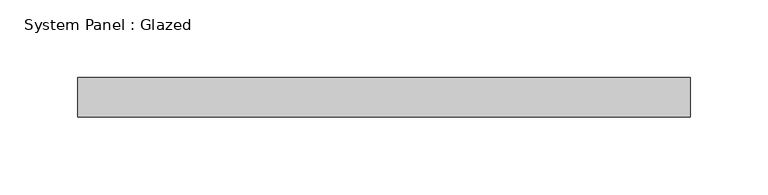
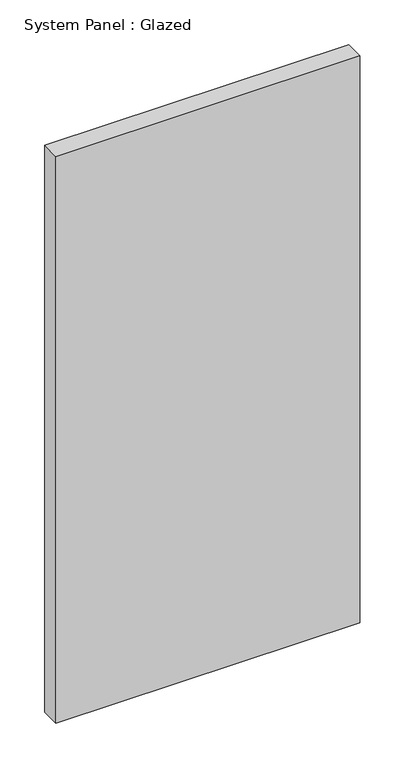
"""IFC4 building model written with IfcOpenShell, lengths in millimetres: plate geometry, System Panel : Glazed."""

from ifc_helpers import new_model, si_unit, origin, origin_with_axes, place, context, project, spatial, polyline, outline, extrude, source, transform, mapped, element, save


def system_panel_glazed_831e08d1(model_context):
    return source(origin(), model_context, "Body", "SweptSolid", [
        extrude(outline(polyline([(196.85, 19.05), (-196.85, 19.05), (-196.85, 44.45), (196.85, 44.45), (196.85, 19.05)])), origin_with_axes(), (0.0, 0.0, 1.0), 776.0351947),
    ])


if __name__ == "__main__":
    model = new_model("IFC4")
    model_context = context("Model", 3, world=origin())
    ifc_project = project(units=[si_unit("LENGTHUNIT", "METRE", prefix="MILLI")], contexts=[model_context])
    site = spatial("IfcSite", under=ifc_project)
    building = spatial("IfcBuilding", under=site)
    placement = place(None, origin())
    system_panel_glazed_shape = system_panel_glazed_831e08d1(model_context)
    element("IfcPlate", 1, ObjectType="System Panel : Glazed", at=placement, inside=building, context=model_context, shape_type="MappedRepresentation", body=[
        mapped(system_panel_glazed_shape, transform((0.0, 0.0, 0.0), x_axis=(1.0, 0.0, 0.0), y_axis=(0.0, 1.0, 0.0), z_axis=(0.0, 0.0, 1.0))),
    ])
    save(model, "model.ifc")

# Revit data of these elements
# Type "System Panel : Glazed"
#   Construction Type Id = "GSP4R"
#   Analytic Construction = "1/8 in Pilkington single glazing"
#   Visual Light Transmittance = 0.9
#   Solar Heat Gain Coefficient = 0.86
#   Heat Transfer Coefficient (U) = 1.18115 BTU/(h·ft²·°F)
#   Define Thermal Properties by = 1
# Element 1 (IfcPlate, "System Panel : Glazed")
#   Materials on its faces: "Glass"
# Materials
#   "Glass": class "Glass", colour RGB 0 128 192, transparency 0.75, Description = "Soda Lime Glass", Cost = 0
